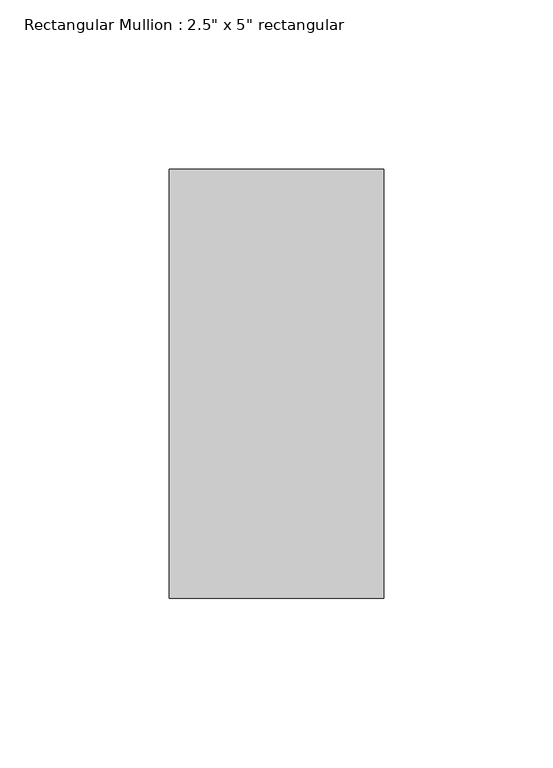
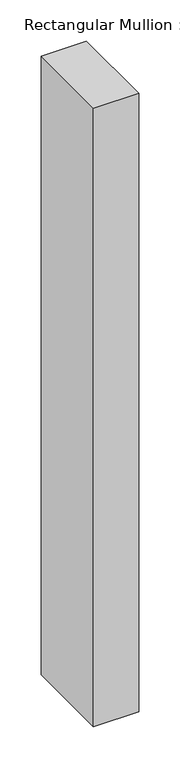
"""IFC4 building model written with IfcOpenShell, lengths in millimetres: member geometry."""

from ifc_helpers import new_model, si_unit, frame, origin, place, context, project, spatial, polyline, outline, extrude, source, transform, mapped, element, save


def member_1d73318e(model_context):
    return source(origin(), model_context, "Body", "SweptSolid", [
        extrude(outline(polyline([(0.0, 63.5), (0.0, -63.5), (-63.5, -63.5), (-63.5, 63.5), (0.0, 63.5)])), frame((0.0, 0.0, -917.1180586), z_axis=(0.0, 0.0, 1.0), x_axis=(1.0, 0.0, 0.0)), (0.0, 0.0, 1.0), 917.1180586),
    ])


if __name__ == "__main__":
    model = new_model("IFC4")
    model_context = context("Model", 3, world=origin())
    ifc_project = project(units=[si_unit("LENGTHUNIT", "METRE", prefix="MILLI")], contexts=[model_context])
    site = spatial("IfcSite", under=ifc_project)
    building = spatial("IfcBuilding", under=site)
    placement = place(None, origin())
    member_shape = member_1d73318e(model_context)
    element("IfcMember", 1, ObjectType="Rectangular Mullion : 2.5\" x 5\" rectangular", at=placement, inside=building, context=model_context, shape_type="MappedRepresentation", body=[
        mapped(member_shape, transform((0.0, 0.0, 0.0), x_axis=(1.0, 0.0, 0.0), y_axis=(0.0, 1.0, 0.0), z_axis=(0.0, 0.0, 1.0))),
    ])
    save(model, "model.ifc")

# Revit data of these elements
# Type "Rectangular Mullion : 2.5\" x 5\" rectangular"
#   built-in parameter 1007304 = 0.416667 (stored number, unit not read)
#   built-in parameter 1007301 = 0.104167 (stored number, unit not read)
#   built-in parameter 1007300 = 0.104167 (stored number, unit not read)
# Element 1 (IfcMember, "Rectangular Mullion : 2.5\" x 5\" rectangular")
#   Materials on its faces: "Aluminum"
# Materials
#   "Aluminum": class "Metal", colour RGB 247 247 247, transparency 0, Description = "Aluminum 6061", Cost = 0
